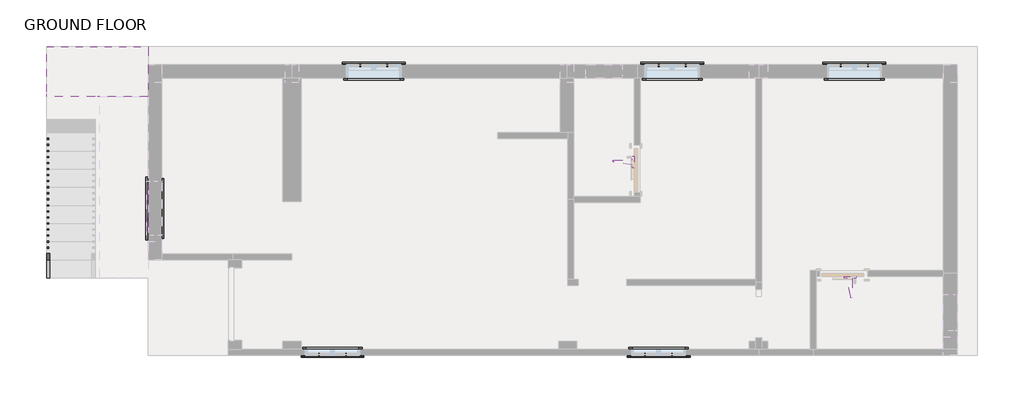
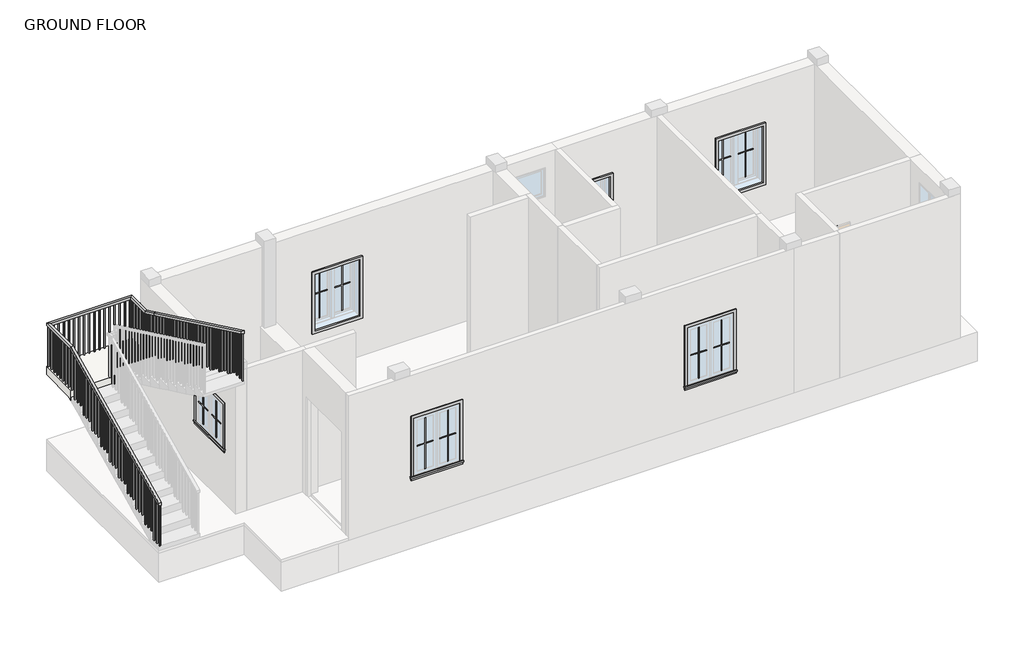
# One storey, part 3 of 3: 26 proxies, 1 railing, 1 slab.
"""IFC4 building model written with IfcOpenShell, lengths in millimetres."""

from ifc_helpers import new_model, si_unit, frame, origin, place, context, project, spatial, polyline, outline, extrude, faceted_brep, transform, mapped, element, save
from components import bel_door_closer_bel_door_closer_f210e2f3, bel_door_closer_bel_door_closer_a3520c2f, muntin_pattern_2x2_muntin_pattern_2x2_1acec82f, muntin_pattern_2x2_muntin_pattern_2x2_43d02eee, muntin_pattern_2x2_muntin_pattern_2x2_d1c6e638, muntin_pattern_2x2_muntin_pattern_2x2_37b95fb2, trim_window_exterior_flat_with_sill_e4b28ec3, trim_window_exterior_flat_with_sill_84e24481, trim_window_interior_flat_picture_frame_39ff4276, trim_window_interior_flat_picture_frame_28d4e5dc

model = new_model("IFC4")

# Units and contexts
model_context = context("Model", 3, world=origin())
ifc_project = project(units=[si_unit("LENGTHUNIT", "METRE", prefix="MILLI")], contexts=[model_context])

# Site, building, storey
site = spatial("IfcSite", under=ifc_project)
building = spatial("IfcBuilding", under=site)
storey = spatial("IfcBuildingStorey", under=building, Name="GROUND FLOOR", Elevation=0.0)

# Proxies
placement = place(None, origin())
bel_door_closer_bel_door_closer_shape = bel_door_closer_bel_door_closer_f210e2f3(model_context)
element("IfcBuildingElementProxy", 1, Name="BEL-Door Closer : BEL-Door Closer", ObjectType="BEL-Door Closer : BEL-Door Closer", at=placement, inside=storey, context=model_context, shape_type="MappedRepresentation", body=[
    mapped(bel_door_closer_bel_door_closer_shape, transform((6826.3533773, 1546.5642852, 2144.6957985), x_axis=(-1.0, 0.0, 0.0), y_axis=(0.0, 0.0, -1.0), z_axis=(0.0, -1.0, 0.0))),
])
bel_door_closer_bel_door_closer_2_shape = bel_door_closer_bel_door_closer_a3520c2f(model_context)
element("IfcBuildingElementProxy", 2, Name="BEL-Door Closer : BEL-Door Closer", ObjectType="BEL-Door Closer : BEL-Door Closer", at=placement, inside=storey, context=model_context, shape_type="MappedRepresentation", body=[
    mapped(bel_door_closer_bel_door_closer_2_shape, transform((3460.0408773, 3211.0767852, 2144.6957985), x_axis=(0.0, -1.0, 0.0), y_axis=(0.0, 0.0, 1.0), z_axis=(-1.0, 0.0, 0.0))),
])
muntin_pattern_2x2_muntin_pattern_2x2_shape = muntin_pattern_2x2_muntin_pattern_2x2_1acec82f(model_context)
element("IfcBuildingElementProxy", 3, Name="Muntin Pattern_2x2 : Muntin Pattern_2x2", ObjectType="Muntin Pattern_2x2 : Muntin Pattern_2x2", at=placement, inside=storey, context=model_context, shape_type="MappedRepresentation", body=[
    mapped(muntin_pattern_2x2_muntin_pattern_2x2_shape, transform((-1135.7716227, 5093.0392852, 984.25), x_axis=(1.0, 0.0, 0.0), y_axis=(0.0, 1.0, 0.0), z_axis=(0.0, 0.0, 1.0))),
])
element("IfcBuildingElementProxy", 4, Name="Muntin Pattern_2x2 : Muntin Pattern_2x2", ObjectType="Muntin Pattern_2x2 : Muntin Pattern_2x2", at=placement, inside=storey, context=model_context, shape_type="MappedRepresentation", body=[
    mapped(muntin_pattern_2x2_muntin_pattern_2x2_shape, transform((3868.0283773, 5093.0392852, 984.25), x_axis=(1.0, 0.0, 0.0), y_axis=(0.0, 1.0, 0.0), z_axis=(0.0, 0.0, 1.0))),
])
element("IfcBuildingElementProxy", 5, Name="Muntin Pattern_2x2 : Muntin Pattern_2x2", ObjectType="Muntin Pattern_2x2 : Muntin Pattern_2x2", at=placement, inside=storey, context=model_context, shape_type="MappedRepresentation", body=[
    mapped(muntin_pattern_2x2_muntin_pattern_2x2_shape, transform((6922.3783773, 5093.0392852, 984.25), x_axis=(1.0, 0.0, 0.0), y_axis=(0.0, 1.0, 0.0), z_axis=(0.0, 0.0, 1.0))),
])
element("IfcBuildingElementProxy", 6, Name="Muntin Pattern_2x2 : Muntin Pattern_2x2", ObjectType="Muntin Pattern_2x2 : Muntin Pattern_2x2", at=placement, inside=storey, context=model_context, shape_type="MappedRepresentation", body=[
    mapped(muntin_pattern_2x2_muntin_pattern_2x2_shape, transform((4093.4533773, 235.2892852, 984.25), x_axis=(-1.0, 0.0, 0.0), y_axis=(0.0, -1.0, 0.0), z_axis=(0.0, 0.0, 1.0))),
])
element("IfcBuildingElementProxy", 7, Name="Muntin Pattern_2x2 : Muntin Pattern_2x2", ObjectType="Muntin Pattern_2x2 : Muntin Pattern_2x2", at=placement, inside=storey, context=model_context, shape_type="MappedRepresentation", body=[
    mapped(muntin_pattern_2x2_muntin_pattern_2x2_shape, transform((-1373.8966227, 235.2892852, 984.25), x_axis=(-1.0, 0.0, 0.0), y_axis=(0.0, -1.0, 0.0), z_axis=(0.0, 0.0, 1.0))),
])
muntin_pattern_2x2_muntin_pattern_2x2_2_shape = muntin_pattern_2x2_muntin_pattern_2x2_43d02eee(model_context)
element("IfcBuildingElementProxy", 8, Name="Muntin Pattern_2x2 : Muntin Pattern_2x2", ObjectType="Muntin Pattern_2x2 : Muntin Pattern_2x2", at=placement, inside=storey, context=model_context, shape_type="MappedRepresentation", body=[
    mapped(muntin_pattern_2x2_muntin_pattern_2x2_2_shape, transform((-681.7466227, 5093.0392852, 984.25), x_axis=(-1.0, 0.0, 0.0), y_axis=(0.0, -1.0, 0.0), z_axis=(0.0, 0.0, 1.0))),
])
element("IfcBuildingElementProxy", 9, Name="Muntin Pattern_2x2 : Muntin Pattern_2x2", ObjectType="Muntin Pattern_2x2 : Muntin Pattern_2x2", at=placement, inside=storey, context=model_context, shape_type="MappedRepresentation", body=[
    mapped(muntin_pattern_2x2_muntin_pattern_2x2_2_shape, transform((4322.0533773, 5093.0392852, 984.25), x_axis=(-1.0, 0.0, 0.0), y_axis=(0.0, -1.0, 0.0), z_axis=(0.0, 0.0, 1.0))),
])
element("IfcBuildingElementProxy", 10, Name="Muntin Pattern_2x2 : Muntin Pattern_2x2", ObjectType="Muntin Pattern_2x2 : Muntin Pattern_2x2", at=placement, inside=storey, context=model_context, shape_type="MappedRepresentation", body=[
    mapped(muntin_pattern_2x2_muntin_pattern_2x2_2_shape, transform((7376.4033773, 5093.0392852, 984.25), x_axis=(-1.0, 0.0, 0.0), y_axis=(0.0, -1.0, 0.0), z_axis=(0.0, 0.0, 1.0))),
])
element("IfcBuildingElementProxy", 11, Name="Muntin Pattern_2x2 : Muntin Pattern_2x2", ObjectType="Muntin Pattern_2x2 : Muntin Pattern_2x2", at=placement, inside=storey, context=model_context, shape_type="MappedRepresentation", body=[
    mapped(muntin_pattern_2x2_muntin_pattern_2x2_2_shape, transform((3639.4283773, 235.2892852, 984.25), x_axis=(1.0, 0.0, 0.0), y_axis=(0.0, 1.0, 0.0), z_axis=(0.0, 0.0, 1.0))),
])
element("IfcBuildingElementProxy", 12, Name="Muntin Pattern_2x2 : Muntin Pattern_2x2", ObjectType="Muntin Pattern_2x2 : Muntin Pattern_2x2", at=placement, inside=storey, context=model_context, shape_type="MappedRepresentation", body=[
    mapped(muntin_pattern_2x2_muntin_pattern_2x2_2_shape, transform((-1827.9216227, 235.2892852, 984.25), x_axis=(1.0, 0.0, 0.0), y_axis=(0.0, 1.0, 0.0), z_axis=(0.0, 0.0, 1.0))),
])
muntin_pattern_2x2_muntin_pattern_2x2_3_shape = muntin_pattern_2x2_muntin_pattern_2x2_d1c6e638(model_context)
element("IfcBuildingElementProxy", 13, Name="Muntin Pattern_2x2 : Muntin Pattern_2x2", ObjectType="Muntin Pattern_2x2 : Muntin Pattern_2x2", at=placement, inside=storey, context=model_context, shape_type="MappedRepresentation", body=[
    mapped(muntin_pattern_2x2_muntin_pattern_2x2_3_shape, transform((-4683.8341227, 2462.5517852, 1289.05), x_axis=(0.0, 1.0, 0.0), y_axis=(-1.0, 0.0, 0.0), z_axis=(0.0, 0.0, 1.0))),
])
muntin_pattern_2x2_muntin_pattern_2x2_4_shape = muntin_pattern_2x2_muntin_pattern_2x2_37b95fb2(model_context)
element("IfcBuildingElementProxy", 14, Name="Muntin Pattern_2x2 : Muntin Pattern_2x2", ObjectType="Muntin Pattern_2x2 : Muntin Pattern_2x2", at=placement, inside=storey, context=model_context, shape_type="MappedRepresentation", body=[
    mapped(muntin_pattern_2x2_muntin_pattern_2x2_4_shape, transform((-4683.8341227, 2916.5767852, 1289.05), x_axis=(0.0, -1.0, 0.0), y_axis=(1.0, 0.0, 0.0), z_axis=(0.0, 0.0, 1.0))),
])
trim_window_exterior_flat_with_sill_shape = trim_window_exterior_flat_with_sill_e4b28ec3(model_context)
element("IfcBuildingElementProxy", 15, Name="Trim-Window-Exterior-Flat : with Sill", ObjectType="Trim-Window-Exterior-Flat : with Sill", at=placement, inside=storey, context=model_context, shape_type="MappedRepresentation", body=[
    mapped(trim_window_exterior_flat_with_sill_shape, transform((-908.7591227, 5102.5642852, 2133.6), x_axis=(-1.0, 0.0, 0.0), y_axis=(0.0, 0.0, 1.0), z_axis=(0.0, 1.0, 0.0))),
])
element("IfcBuildingElementProxy", 16, Name="Trim-Window-Exterior-Flat : with Sill", ObjectType="Trim-Window-Exterior-Flat : with Sill", at=placement, inside=storey, context=model_context, shape_type="MappedRepresentation", body=[
    mapped(trim_window_exterior_flat_with_sill_shape, transform((4095.0408773, 5102.5642852, 2133.6), x_axis=(-1.0, 0.0, 0.0), y_axis=(0.0, 0.0, 1.0), z_axis=(0.0, 1.0, 0.0))),
])
element("IfcBuildingElementProxy", 17, Name="Trim-Window-Exterior-Flat : with Sill", ObjectType="Trim-Window-Exterior-Flat : with Sill", at=placement, inside=storey, context=model_context, shape_type="MappedRepresentation", body=[
    mapped(trim_window_exterior_flat_with_sill_shape, transform((7149.3908773, 5102.5642852, 2133.6), x_axis=(-1.0, 0.0, 0.0), y_axis=(0.0, 0.0, 1.0), z_axis=(0.0, 1.0, 0.0))),
])
element("IfcBuildingElementProxy", 18, Name="Trim-Window-Exterior-Flat : with Sill", ObjectType="Trim-Window-Exterior-Flat : with Sill", at=placement, inside=storey, context=model_context, shape_type="MappedRepresentation", body=[
    mapped(trim_window_exterior_flat_with_sill_shape, transform((3866.4408773, 225.7642852, 2133.6), x_axis=(1.0, 0.0, 0.0), y_axis=(0.0, 0.0, 1.0), z_axis=(0.0, -1.0, 0.0))),
])
element("IfcBuildingElementProxy", 19, Name="Trim-Window-Exterior-Flat : with Sill", ObjectType="Trim-Window-Exterior-Flat : with Sill", at=placement, inside=storey, context=model_context, shape_type="MappedRepresentation", body=[
    mapped(trim_window_exterior_flat_with_sill_shape, transform((-1600.9091227, 225.7642852, 2133.6), x_axis=(1.0, 0.0, 0.0), y_axis=(0.0, 0.0, 1.0), z_axis=(0.0, -1.0, 0.0))),
])
trim_window_exterior_flat_with_sill_2_shape = trim_window_exterior_flat_with_sill_84e24481(model_context)
element("IfcBuildingElementProxy", 20, Name="Trim-Window-Exterior-Flat : with Sill", ObjectType="Trim-Window-Exterior-Flat : with Sill", at=placement, inside=storey, context=model_context, shape_type="MappedRepresentation", body=[
    mapped(trim_window_exterior_flat_with_sill_2_shape, transform((-4693.3591227, 2689.5642852, 2133.6), x_axis=(0.0, -1.0, 0.0), y_axis=(0.0, 0.0, 1.0), z_axis=(-1.0, 0.0, 0.0))),
])
trim_window_interior_flat_picture_frame_shape = trim_window_interior_flat_picture_frame_39ff4276(model_context)
element("IfcBuildingElementProxy", 21, Name="Trim-Window-Interior-Flat : Picture Frame", ObjectType="Trim-Window-Interior-Flat : Picture Frame", at=placement, inside=storey, context=model_context, shape_type="MappedRepresentation", body=[
    mapped(trim_window_interior_flat_picture_frame_shape, transform((-908.7591227, 4873.9642852, 2133.6), x_axis=(1.0, 0.0, 0.0), y_axis=(0.0, 0.0, 1.0), z_axis=(0.0, -1.0, 0.0))),
])
element("IfcBuildingElementProxy", 22, Name="Trim-Window-Interior-Flat : Picture Frame", ObjectType="Trim-Window-Interior-Flat : Picture Frame", at=placement, inside=storey, context=model_context, shape_type="MappedRepresentation", body=[
    mapped(trim_window_interior_flat_picture_frame_shape, transform((4095.0408773, 4873.9642852, 2133.6), x_axis=(1.0, 0.0, 0.0), y_axis=(0.0, 0.0, 1.0), z_axis=(0.0, -1.0, 0.0))),
])
element("IfcBuildingElementProxy", 23, Name="Trim-Window-Interior-Flat : Picture Frame", ObjectType="Trim-Window-Interior-Flat : Picture Frame", at=placement, inside=storey, context=model_context, shape_type="MappedRepresentation", body=[
    mapped(trim_window_interior_flat_picture_frame_shape, transform((7149.3908773, 4873.9642852, 2133.6), x_axis=(1.0, 0.0, 0.0), y_axis=(0.0, 0.0, 1.0), z_axis=(0.0, -1.0, 0.0))),
])
element("IfcBuildingElementProxy", 24, Name="Trim-Window-Interior-Flat : Picture Frame", ObjectType="Trim-Window-Interior-Flat : Picture Frame", at=placement, inside=storey, context=model_context, shape_type="MappedRepresentation", body=[
    mapped(trim_window_interior_flat_picture_frame_shape, transform((3866.4408773, 327.3642852, 2133.6), x_axis=(-1.0, 0.0, 0.0), y_axis=(0.0, 0.0, 1.0), z_axis=(0.0, 1.0, 0.0))),
])
element("IfcBuildingElementProxy", 25, Name="Trim-Window-Interior-Flat : Picture Frame", ObjectType="Trim-Window-Interior-Flat : Picture Frame", at=placement, inside=storey, context=model_context, shape_type="MappedRepresentation", body=[
    mapped(trim_window_interior_flat_picture_frame_shape, transform((-1600.9091227, 327.3642852, 2133.6), x_axis=(-1.0, 0.0, 0.0), y_axis=(0.0, 0.0, 1.0), z_axis=(0.0, 1.0, 0.0))),
])
trim_window_interior_flat_picture_frame_2_shape = trim_window_interior_flat_picture_frame_28d4e5dc(model_context)
element("IfcBuildingElementProxy", 26, Name="Trim-Window-Interior-Flat : Picture Frame", ObjectType="Trim-Window-Interior-Flat : Picture Frame", at=placement, inside=storey, context=model_context, shape_type="MappedRepresentation", body=[
    mapped(trim_window_interior_flat_picture_frame_2_shape, transform((-4464.7591227, 2689.5642852, 2133.6), x_axis=(0.0, 1.0, 0.0), y_axis=(0.0, 0.0, 1.0), z_axis=(1.0, 0.0, 0.0))),
])

# Railing
element("IfcRailing", 27, ObjectType="Handrail - Rectangular", at=placement, inside=storey, context=model_context, shape_type="SolidModel", body=[
    faceted_brep([(-6395.1591227, 1521.1642852, 1059.8727273), (-6395.1591227, 1521.1642852, 1003.5834559), (-6344.3591227, 1521.1642852, 1003.5834559), (-6344.3591227, 1521.1642852, 1059.8727273), (-6395.1591227, 4569.1642852, 2514.6), (-6395.1591227, 4580.6656156, 2463.8), (-6344.3591227, 4580.6656156, 2463.8), (-6344.3591227, 4569.1642852, 2514.6), (-6395.1591227, 5407.3642852, 2514.6), (-6395.1591227, 5407.3642852, 2463.8), (-6344.3591227, 5356.5642852, 2463.8), (-6344.3591227, 5356.5642852, 2514.6), (-4693.3591227, 5407.3642852, 2514.6), (-4693.3591227, 5407.3642852, 2463.8), (-4744.1591227, 5356.5642852, 2463.8), (-4744.1591227, 5356.5642852, 2514.6), (-4693.3591227, 4873.9642852, 2514.6), (-4693.3591227, 4862.4629548, 2463.8), (-4744.1591227, 4862.4629548, 2463.8), (-4744.1591227, 4873.9642852, 2514.6), (-4693.3591227, 4569.1642852, 2660.0727273), (-4693.3591227, 4547.2832222, 2614.2266906), (-4744.1591227, 4547.2832222, 2614.2266906), (-4744.1591227, 4569.1642852, 2660.0727273), (-4693.3591227, 1521.1642852, 4114.8), (-4744.1591227, 1521.1642852, 4114.8), (-4744.1591227, 1521.1642852, 4058.5107287), (-4693.3591227, 1521.1642852, 4058.5107287)], [[[0, 1, 2, 3]], [[1, 0, 4, 5]], [[2, 1, 5, 6]], [[3, 2, 6, 7]], [[0, 3, 7, 4]], [[5, 4, 8, 9]], [[6, 5, 9, 10]], [[7, 6, 10, 11]], [[4, 7, 11, 8]], [[9, 8, 12, 13]], [[10, 9, 13, 14]], [[11, 10, 14, 15]], [[8, 11, 15, 12]], [[13, 12, 16, 17]], [[14, 13, 17, 18]], [[15, 14, 18, 19]], [[12, 15, 19, 16]], [[17, 16, 20, 21]], [[18, 17, 21, 22]], [[19, 18, 22, 23]], [[16, 19, 23, 20]], [[24, 25, 26, 27]], [[21, 20, 24, 27]], [[22, 21, 27, 26]], [[23, 22, 26, 25]], [[20, 23, 25, 24]]]),
    extrude(outline(polyline([(1632.2892852, 4005.4737969), (1632.2892852, 3054.9272727), (1613.2392852, 3054.9272727), (1613.2392852, 4014.5658423), (1632.2892852, 4005.4737969)])), frame((-4728.2841227, 0.0, 0.0), z_axis=(1.0, 0.0, 0.0), x_axis=(0.0, 1.0, 0.0)), (0.0, 0.0, 1.0), 19.05),
    extrude(outline(polyline([(1733.8892852, 3956.9828878), (1733.8892852, 3054.9272727), (1714.8392852, 3054.9272727), (1714.8392852, 3966.0749332), (1733.8892852, 3956.9828878)])), frame((-4728.2841227, 0.0, 0.0), z_axis=(1.0, 0.0, 0.0), x_axis=(0.0, 1.0, 0.0)), (0.0, 0.0, 1.0), 19.05),
    extrude(outline(polyline([(1835.4892852, 3908.4919787), (1835.4892852, 3054.9272727), (1816.4392852, 3054.9272727), (1816.4392852, 3917.5840241), (1835.4892852, 3908.4919787)])), frame((-4728.2841227, 0.0, 0.0), z_axis=(1.0, 0.0, 0.0), x_axis=(0.0, 1.0, 0.0)), (0.0, 0.0, 1.0), 19.05),
    extrude(outline(polyline([(1937.0892852, 3860.0010696), (1937.0892852, 2909.4545455), (1918.0392852, 2909.4545455), (1918.0392852, 3869.093115), (1937.0892852, 3860.0010696)])), frame((-4728.2841227, 0.0, 0.0), z_axis=(1.0, 0.0, 0.0), x_axis=(0.0, 1.0, 0.0)), (0.0, 0.0, 1.0), 19.05),
    extrude(outline(polyline([(2038.6892852, 3811.5101605), (2038.6892852, 2909.4545455), (2019.6392852, 2909.4545455), (2019.6392852, 3820.6022059), (2038.6892852, 3811.5101605)])), frame((-4728.2841227, 0.0, 0.0), z_axis=(1.0, 0.0, 0.0), x_axis=(0.0, 1.0, 0.0)), (0.0, 0.0, 1.0), 19.05),
    extrude(outline(polyline([(2140.2892852, 3763.0192514), (2140.2892852, 2909.4545455), (2121.2392852, 2909.4545455), (2121.2392852, 3772.1112969), (2140.2892852, 3763.0192514)])), frame((-4728.2841227, 0.0, 0.0), z_axis=(1.0, 0.0, 0.0), x_axis=(0.0, 1.0, 0.0)), (0.0, 0.0, 1.0), 19.05),
    extrude(outline(polyline([(2241.8892852, 3714.5283423), (2241.8892852, 2763.9818182), (2222.8392852, 2763.9818182), (2222.8392852, 3723.6203878), (2241.8892852, 3714.5283423)])), frame((-4728.2841227, 0.0, 0.0), z_axis=(1.0, 0.0, 0.0), x_axis=(0.0, 1.0, 0.0)), (0.0, 0.0, 1.0), 19.05),
    extrude(outline(polyline([(2343.4892852, 3666.0374332), (2343.4892852, 2763.9818182), (2324.4392852, 2763.9818182), (2324.4392852, 3675.1294787), (2343.4892852, 3666.0374332)])), frame((-4728.2841227, 0.0, 0.0), z_axis=(1.0, 0.0, 0.0), x_axis=(0.0, 1.0, 0.0)), (0.0, 0.0, 1.0), 19.05),
    extrude(outline(polyline([(2445.0892852, 3617.5465241), (2445.0892852, 2763.9818182), (2426.0392852, 2763.9818182), (2426.0392852, 3626.6385696), (2445.0892852, 3617.5465241)])), frame((-4728.2841227, 0.0, 0.0), z_axis=(1.0, 0.0, 0.0), x_axis=(0.0, 1.0, 0.0)), (0.0, 0.0, 1.0), 19.05),
    extrude(outline(polyline([(2546.6892852, 3569.055615), (2546.6892852, 2618.5090909), (2527.6392852, 2618.5090909), (2527.6392852, 3578.1476605), (2546.6892852, 3569.055615)])), frame((-4728.2841227, 0.0, 0.0), z_axis=(1.0, 0.0, 0.0), x_axis=(0.0, 1.0, 0.0)), (0.0, 0.0, 1.0), 19.05),
    extrude(outline(polyline([(2648.2892852, 3520.5647059), (2648.2892852, 2618.5090909), (2629.2392852, 2618.5090909), (2629.2392852, 3529.6567514), (2648.2892852, 3520.5647059)])), frame((-4728.2841227, 0.0, 0.0), z_axis=(1.0, 0.0, 0.0), x_axis=(0.0, 1.0, 0.0)), (0.0, 0.0, 1.0), 19.05),
    extrude(outline(polyline([(2749.8892852, 3472.0737969), (2749.8892852, 2618.5090909), (2730.8392852, 2618.5090909), (2730.8392852, 3481.1658423), (2749.8892852, 3472.0737969)])), frame((-4728.2841227, 0.0, 0.0), z_axis=(1.0, 0.0, 0.0), x_axis=(0.0, 1.0, 0.0)), (0.0, 0.0, 1.0), 19.05),
    extrude(outline(polyline([(2851.4892852, 3423.5828878), (2851.4892852, 2473.0363636), (2832.4392852, 2473.0363636), (2832.4392852, 3432.6749332), (2851.4892852, 3423.5828878)])), frame((-4728.2841227, 0.0, 0.0), z_axis=(1.0, 0.0, 0.0), x_axis=(0.0, 1.0, 0.0)), (0.0, 0.0, 1.0), 19.05),
    extrude(outline(polyline([(2953.0892852, 3375.0919787), (2953.0892852, 2473.0363636), (2934.0392852, 2473.0363636), (2934.0392852, 3384.1840241), (2953.0892852, 3375.0919787)])), frame((-4728.2841227, 0.0, 0.0), z_axis=(1.0, 0.0, 0.0), x_axis=(0.0, 1.0, 0.0)), (0.0, 0.0, 1.0), 19.05),
    extrude(outline(polyline([(3054.6892852, 3326.6010696), (3054.6892852, 2473.0363636), (3035.6392852, 2473.0363636), (3035.6392852, 3335.693115), (3054.6892852, 3326.6010696)])), frame((-4728.2841227, 0.0, 0.0), z_axis=(1.0, 0.0, 0.0), x_axis=(0.0, 1.0, 0.0)), (0.0, 0.0, 1.0), 19.05),
    extrude(outline(polyline([(3156.2892852, 3278.1101605), (3156.2892852, 2327.5636364), (3137.2392852, 2327.5636364), (3137.2392852, 3287.2022059), (3156.2892852, 3278.1101605)])), frame((-4728.2841227, 0.0, 0.0), z_axis=(1.0, 0.0, 0.0), x_axis=(0.0, 1.0, 0.0)), (0.0, 0.0, 1.0), 19.05),
    extrude(outline(polyline([(3257.8892852, 3229.6192514), (3257.8892852, 2327.5636364), (3238.8392852, 2327.5636364), (3238.8392852, 3238.7112969), (3257.8892852, 3229.6192514)])), frame((-4728.2841227, 0.0, 0.0), z_axis=(1.0, 0.0, 0.0), x_axis=(0.0, 1.0, 0.0)), (0.0, 0.0, 1.0), 19.05),
    extrude(outline(polyline([(3359.4892852, 3181.1283423), (3359.4892852, 2327.5636364), (3340.4392852, 2327.5636364), (3340.4392852, 3190.2203878), (3359.4892852, 3181.1283423)])), frame((-4728.2841227, 0.0, 0.0), z_axis=(1.0, 0.0, 0.0), x_axis=(0.0, 1.0, 0.0)), (0.0, 0.0, 1.0), 19.05),
    extrude(outline(polyline([(3461.0892852, 3132.6374332), (3461.0892852, 2182.0909091), (3442.0392852, 2182.0909091), (3442.0392852, 3141.7294787), (3461.0892852, 3132.6374332)])), frame((-4728.2841227, 0.0, 0.0), z_axis=(1.0, 0.0, 0.0), x_axis=(0.0, 1.0, 0.0)), (0.0, 0.0, 1.0), 19.05),
    extrude(outline(polyline([(3562.6892852, 3084.1465241), (3562.6892852, 2182.0909091), (3543.6392852, 2182.0909091), (3543.6392852, 3093.2385696), (3562.6892852, 3084.1465241)])), frame((-4728.2841227, 0.0, 0.0), z_axis=(1.0, 0.0, 0.0), x_axis=(0.0, 1.0, 0.0)), (0.0, 0.0, 1.0), 19.05),
    extrude(outline(polyline([(3664.2892852, 3035.655615), (3664.2892852, 2182.0909091), (3645.2392852, 2182.0909091), (3645.2392852, 3044.7476605), (3664.2892852, 3035.655615)])), frame((-4728.2841227, 0.0, 0.0), z_axis=(1.0, 0.0, 0.0), x_axis=(0.0, 1.0, 0.0)), (0.0, 0.0, 1.0), 19.05),
    extrude(outline(polyline([(3765.8892852, 2987.1647059), (3765.8892852, 2036.6181818), (3746.8392852, 2036.6181818), (3746.8392852, 2996.2567514), (3765.8892852, 2987.1647059)])), frame((-4728.2841227, 0.0, 0.0), z_axis=(1.0, 0.0, 0.0), x_axis=(0.0, 1.0, 0.0)), (0.0, 0.0, 1.0), 19.05),
    extrude(outline(polyline([(3867.4892852, 2938.6737969), (3867.4892852, 2036.6181818), (3848.4392852, 2036.6181818), (3848.4392852, 2947.7658423), (3867.4892852, 2938.6737969)])), frame((-4728.2841227, 0.0, 0.0), z_axis=(1.0, 0.0, 0.0), x_axis=(0.0, 1.0, 0.0)), (0.0, 0.0, 1.0), 19.05),
    extrude(outline(polyline([(3969.0892852, 2890.1828878), (3969.0892852, 2036.6181818), (3950.0392852, 2036.6181818), (3950.0392852, 2899.2749332), (3969.0892852, 2890.1828878)])), frame((-4728.2841227, 0.0, 0.0), z_axis=(1.0, 0.0, 0.0), x_axis=(0.0, 1.0, 0.0)), (0.0, 0.0, 1.0), 19.05),
    extrude(outline(polyline([(4070.6892852, 2841.6919787), (4070.6892852, 1891.1454545), (4051.6392852, 1891.1454545), (4051.6392852, 2850.7840241), (4070.6892852, 2841.6919787)])), frame((-4728.2841227, 0.0, 0.0), z_axis=(1.0, 0.0, 0.0), x_axis=(0.0, 1.0, 0.0)), (0.0, 0.0, 1.0), 19.05),
    extrude(outline(polyline([(4172.2892852, 2793.2010696), (4172.2892852, 1891.1454545), (4153.2392852, 1891.1454545), (4153.2392852, 2802.293115), (4172.2892852, 2793.2010696)])), frame((-4728.2841227, 0.0, 0.0), z_axis=(1.0, 0.0, 0.0), x_axis=(0.0, 1.0, 0.0)), (0.0, 0.0, 1.0), 19.05),
    extrude(outline(polyline([(4273.8892852, 2744.7101605), (4273.8892852, 1891.1454545), (4254.8392852, 1891.1454545), (4254.8392852, 2753.8022059), (4273.8892852, 2744.7101605)])), frame((-4728.2841227, 0.0, 0.0), z_axis=(1.0, 0.0, 0.0), x_axis=(0.0, 1.0, 0.0)), (0.0, 0.0, 1.0), 19.05),
    extrude(outline(polyline([(4375.4892852, 2696.2192514), (4375.4892852, 1745.6727273), (4356.4392852, 1745.6727273), (4356.4392852, 2705.3112969), (4375.4892852, 2696.2192514)])), frame((-4728.2841227, 0.0, 0.0), z_axis=(1.0, 0.0, 0.0), x_axis=(0.0, 1.0, 0.0)), (0.0, 0.0, 1.0), 19.05),
    extrude(outline(polyline([(4477.0892852, 2647.7283423), (4477.0892852, 1745.6727273), (4458.0392852, 1745.6727273), (4458.0392852, 2656.8203878), (4477.0892852, 2647.7283423)])), frame((-4728.2841227, 0.0, 0.0), z_axis=(1.0, 0.0, 0.0), x_axis=(0.0, 1.0, 0.0)), (0.0, 0.0, 1.0), 19.05),
    extrude(outline(polyline([(4680.2892852, 2550.7465241), (4680.2892852, 1600.2), (4661.2392852, 1600.2), (4661.2392852, 2559.8385696), (4680.2892852, 2550.7465241)])), frame((-4728.2841227, 0.0, 0.0), z_axis=(1.0, 0.0, 0.0), x_axis=(0.0, 1.0, 0.0)), (0.0, 0.0, 1.0), 19.05),
    extrude(outline(polyline([(4781.8892852, 2502.255615), (4781.8892852, 1600.2), (4762.8392852, 1600.2), (4762.8392852, 2511.3476605), (4781.8892852, 2502.255615)])), frame((-4728.2841227, 0.0, 0.0), z_axis=(1.0, 0.0, 0.0), x_axis=(0.0, 1.0, 0.0)), (0.0, 0.0, 1.0), 19.05),
    extrude(outline(polyline([(-4709.2341227, 4883.4892852), (-4709.2341227, 4864.4392852), (-4728.2841227, 4864.4392852), (-4728.2841227, 4883.4892852), (-4709.2341227, 4883.4892852)])), frame((0.0, 0.0, 1600.2), z_axis=(0.0, 0.0, 1.0), x_axis=(1.0, 0.0, 0.0)), (0.0, 0.0, 1.0), 863.6),
    extrude(outline(polyline([(-4709.2341227, 4985.0892852), (-4709.2341227, 4966.0392852), (-4728.2841227, 4966.0392852), (-4728.2841227, 4985.0892852), (-4709.2341227, 4985.0892852)])), frame((0.0, 0.0, 1600.2), z_axis=(0.0, 0.0, 1.0), x_axis=(1.0, 0.0, 0.0)), (0.0, 0.0, 1.0), 863.6),
    extrude(outline(polyline([(-4709.2341227, 5086.6892852), (-4709.2341227, 5067.6392852), (-4728.2841227, 5067.6392852), (-4728.2841227, 5086.6892852), (-4709.2341227, 5086.6892852)])), frame((0.0, 0.0, 1600.2), z_axis=(0.0, 0.0, 1.0), x_axis=(1.0, 0.0, 0.0)), (0.0, 0.0, 1.0), 863.6),
    extrude(outline(polyline([(-4709.2341227, 5188.2892852), (-4709.2341227, 5169.2392852), (-4728.2841227, 5169.2392852), (-4728.2841227, 5188.2892852), (-4709.2341227, 5188.2892852)])), frame((0.0, 0.0, 1600.2), z_axis=(0.0, 0.0, 1.0), x_axis=(1.0, 0.0, 0.0)), (0.0, 0.0, 1.0), 863.6),
    extrude(outline(polyline([(-4709.2341227, 5289.8892852), (-4709.2341227, 5270.8392852), (-4728.2841227, 5270.8392852), (-4728.2841227, 5289.8892852), (-4709.2341227, 5289.8892852)])), frame((0.0, 0.0, 1600.2), z_axis=(0.0, 0.0, 1.0), x_axis=(1.0, 0.0, 0.0)), (0.0, 0.0, 1.0), 863.6),
    extrude(outline(polyline([(-4753.6841227, 5391.4892852), (-4734.6341227, 5391.4892852), (-4734.6341227, 5372.4392852), (-4753.6841227, 5372.4392852), (-4753.6841227, 5391.4892852)])), frame((0.0, 0.0, 1600.2), z_axis=(0.0, 0.0, 1.0), x_axis=(1.0, 0.0, 0.0)), (0.0, 0.0, 1.0), 863.6),
    extrude(outline(polyline([(-4855.2841227, 5391.4892852), (-4836.2341227, 5391.4892852), (-4836.2341227, 5372.4392852), (-4855.2841227, 5372.4392852), (-4855.2841227, 5391.4892852)])), frame((0.0, 0.0, 1600.2), z_axis=(0.0, 0.0, 1.0), x_axis=(1.0, 0.0, 0.0)), (0.0, 0.0, 1.0), 863.6),
    extrude(outline(polyline([(-4956.8841227, 5391.4892852), (-4937.8341227, 5391.4892852), (-4937.8341227, 5372.4392852), (-4956.8841227, 5372.4392852), (-4956.8841227, 5391.4892852)])), frame((0.0, 0.0, 1600.2), z_axis=(0.0, 0.0, 1.0), x_axis=(1.0, 0.0, 0.0)), (0.0, 0.0, 1.0), 863.6),
    extrude(outline(polyline([(-5058.4841227, 5391.4892852), (-5039.4341227, 5391.4892852), (-5039.4341227, 5372.4392852), (-5058.4841227, 5372.4392852), (-5058.4841227, 5391.4892852)])), frame((0.0, 0.0, 1600.2), z_axis=(0.0, 0.0, 1.0), x_axis=(1.0, 0.0, 0.0)), (0.0, 0.0, 1.0), 863.6),
    extrude(outline(polyline([(-5160.0841227, 5391.4892852), (-5141.0341227, 5391.4892852), (-5141.0341227, 5372.4392852), (-5160.0841227, 5372.4392852), (-5160.0841227, 5391.4892852)])), frame((0.0, 0.0, 1600.2), z_axis=(0.0, 0.0, 1.0), x_axis=(1.0, 0.0, 0.0)), (0.0, 0.0, 1.0), 863.6),
    extrude(outline(polyline([(-5261.6841227, 5391.4892852), (-5242.6341227, 5391.4892852), (-5242.6341227, 5372.4392852), (-5261.6841227, 5372.4392852), (-5261.6841227, 5391.4892852)])), frame((0.0, 0.0, 1600.2), z_axis=(0.0, 0.0, 1.0), x_axis=(1.0, 0.0, 0.0)), (0.0, 0.0, 1.0), 863.6),
    extrude(outline(polyline([(-5363.2841227, 5391.4892852), (-5344.2341227, 5391.4892852), (-5344.2341227, 5372.4392852), (-5363.2841227, 5372.4392852), (-5363.2841227, 5391.4892852)])), frame((0.0, 0.0, 1600.2), z_axis=(0.0, 0.0, 1.0), x_axis=(1.0, 0.0, 0.0)), (0.0, 0.0, 1.0), 863.6),
    extrude(outline(polyline([(-5464.8841227, 5391.4892852), (-5445.8341227, 5391.4892852), (-5445.8341227, 5372.4392852), (-5464.8841227, 5372.4392852), (-5464.8841227, 5391.4892852)])), frame((0.0, 0.0, 1600.2), z_axis=(0.0, 0.0, 1.0), x_axis=(1.0, 0.0, 0.0)), (0.0, 0.0, 1.0), 863.6),
    extrude(outline(polyline([(-5566.4841227, 5391.4892852), (-5547.4341227, 5391.4892852), (-5547.4341227, 5372.4392852), (-5566.4841227, 5372.4392852), (-5566.4841227, 5391.4892852)])), frame((0.0, 0.0, 1600.2), z_axis=(0.0, 0.0, 1.0), x_axis=(1.0, 0.0, 0.0)), (0.0, 0.0, 1.0), 863.6),
    extrude(outline(polyline([(-5668.0841227, 5391.4892852), (-5649.0341227, 5391.4892852), (-5649.0341227, 5372.4392852), (-5668.0841227, 5372.4392852), (-5668.0841227, 5391.4892852)])), frame((0.0, 0.0, 1600.2), z_axis=(0.0, 0.0, 1.0), x_axis=(1.0, 0.0, 0.0)), (0.0, 0.0, 1.0), 863.6),
    extrude(outline(polyline([(-5769.6841227, 5391.4892852), (-5750.6341227, 5391.4892852), (-5750.6341227, 5372.4392852), (-5769.6841227, 5372.4392852), (-5769.6841227, 5391.4892852)])), frame((0.0, 0.0, 1600.2), z_axis=(0.0, 0.0, 1.0), x_axis=(1.0, 0.0, 0.0)), (0.0, 0.0, 1.0), 863.6),
    extrude(outline(polyline([(-5871.2841227, 5391.4892852), (-5852.2341227, 5391.4892852), (-5852.2341227, 5372.4392852), (-5871.2841227, 5372.4392852), (-5871.2841227, 5391.4892852)])), frame((0.0, 0.0, 1600.2), z_axis=(0.0, 0.0, 1.0), x_axis=(1.0, 0.0, 0.0)), (0.0, 0.0, 1.0), 863.6),
    extrude(outline(polyline([(-5972.8841227, 5391.4892852), (-5953.8341227, 5391.4892852), (-5953.8341227, 5372.4392852), (-5972.8841227, 5372.4392852), (-5972.8841227, 5391.4892852)])), frame((0.0, 0.0, 1600.2), z_axis=(0.0, 0.0, 1.0), x_axis=(1.0, 0.0, 0.0)), (0.0, 0.0, 1.0), 863.6),
    extrude(outline(polyline([(-6074.4841227, 5391.4892852), (-6055.4341227, 5391.4892852), (-6055.4341227, 5372.4392852), (-6074.4841227, 5372.4392852), (-6074.4841227, 5391.4892852)])), frame((0.0, 0.0, 1600.2), z_axis=(0.0, 0.0, 1.0), x_axis=(1.0, 0.0, 0.0)), (0.0, 0.0, 1.0), 863.6),
    extrude(outline(polyline([(-6176.0841227, 5391.4892852), (-6157.0341227, 5391.4892852), (-6157.0341227, 5372.4392852), (-6176.0841227, 5372.4392852), (-6176.0841227, 5391.4892852)])), frame((0.0, 0.0, 1600.2), z_axis=(0.0, 0.0, 1.0), x_axis=(1.0, 0.0, 0.0)), (0.0, 0.0, 1.0), 863.6),
    extrude(outline(polyline([(-6277.6841227, 5391.4892852), (-6258.6341227, 5391.4892852), (-6258.6341227, 5372.4392852), (-6277.6841227, 5372.4392852), (-6277.6841227, 5391.4892852)])), frame((0.0, 0.0, 1600.2), z_axis=(0.0, 0.0, 1.0), x_axis=(1.0, 0.0, 0.0)), (0.0, 0.0, 1.0), 863.6),
    extrude(outline(polyline([(-6379.2841227, 5270.8392852), (-6379.2841227, 5289.8892852), (-6360.2341227, 5289.8892852), (-6360.2341227, 5270.8392852), (-6379.2841227, 5270.8392852)])), frame((0.0, 0.0, 1600.2), z_axis=(0.0, 0.0, 1.0), x_axis=(1.0, 0.0, 0.0)), (0.0, 0.0, 1.0), 863.6),
    extrude(outline(polyline([(-6379.2841227, 5169.2392852), (-6379.2841227, 5188.2892852), (-6360.2341227, 5188.2892852), (-6360.2341227, 5169.2392852), (-6379.2841227, 5169.2392852)])), frame((0.0, 0.0, 1600.2), z_axis=(0.0, 0.0, 1.0), x_axis=(1.0, 0.0, 0.0)), (0.0, 0.0, 1.0), 863.6),
    extrude(outline(polyline([(-6379.2841227, 5067.6392852), (-6379.2841227, 5086.6892852), (-6360.2341227, 5086.6892852), (-6360.2341227, 5067.6392852), (-6379.2841227, 5067.6392852)])), frame((0.0, 0.0, 1600.2), z_axis=(0.0, 0.0, 1.0), x_axis=(1.0, 0.0, 0.0)), (0.0, 0.0, 1.0), 863.6),
    extrude(outline(polyline([(-6379.2841227, 4966.0392852), (-6379.2841227, 4985.0892852), (-6360.2341227, 4985.0892852), (-6360.2341227, 4966.0392852), (-6379.2841227, 4966.0392852)])), frame((0.0, 0.0, 1600.2), z_axis=(0.0, 0.0, 1.0), x_axis=(1.0, 0.0, 0.0)), (0.0, 0.0, 1.0), 863.6),
    extrude(outline(polyline([(-6379.2841227, 4864.4392852), (-6379.2841227, 4883.4892852), (-6360.2341227, 4883.4892852), (-6360.2341227, 4864.4392852), (-6379.2841227, 4864.4392852)])), frame((0.0, 0.0, 1600.2), z_axis=(0.0, 0.0, 1.0), x_axis=(1.0, 0.0, 0.0)), (0.0, 0.0, 1.0), 863.6),
    extrude(outline(polyline([(-6379.2841227, 4762.8392852), (-6379.2841227, 4781.8892852), (-6360.2341227, 4781.8892852), (-6360.2341227, 4762.8392852), (-6379.2841227, 4762.8392852)])), frame((0.0, 0.0, 1600.2), z_axis=(0.0, 0.0, 1.0), x_axis=(1.0, 0.0, 0.0)), (0.0, 0.0, 1.0), 863.6),
    extrude(outline(polyline([(-6379.2841227, 4661.2392852), (-6379.2841227, 4680.2892852), (-6360.2341227, 4680.2892852), (-6360.2341227, 4661.2392852), (-6379.2841227, 4661.2392852)])), frame((0.0, 0.0, 1600.2), z_axis=(0.0, 0.0, 1.0), x_axis=(1.0, 0.0, 0.0)), (0.0, 0.0, 1.0), 863.6),
    extrude(outline(polyline([(4477.0892852, 2414.3658423), (4477.0892852, 1454.7272727), (4458.0392852, 1454.7272727), (4458.0392852, 2405.2737969), (4477.0892852, 2414.3658423)])), frame((-6379.2841227, 0.0, 0.0), z_axis=(1.0, 0.0, 0.0), x_axis=(0.0, 1.0, 0.0)), (0.0, 0.0, 1.0), 19.05),
    extrude(outline(polyline([(4375.4892852, 2365.8749332), (4375.4892852, 1454.7272727), (4356.4392852, 1454.7272727), (4356.4392852, 2356.7828878), (4375.4892852, 2365.8749332)])), frame((-6379.2841227, 0.0, 0.0), z_axis=(1.0, 0.0, 0.0), x_axis=(0.0, 1.0, 0.0)), (0.0, 0.0, 1.0), 19.05),
    extrude(outline(polyline([(4273.8892852, 2317.3840241), (4273.8892852, 1454.7272727), (4254.8392852, 1454.7272727), (4254.8392852, 2308.2919787), (4273.8892852, 2317.3840241)])), frame((-6379.2841227, 0.0, 0.0), z_axis=(1.0, 0.0, 0.0), x_axis=(0.0, 1.0, 0.0)), (0.0, 0.0, 1.0), 19.05),
    extrude(outline(polyline([(4172.2892852, 2268.893115), (4172.2892852, 1309.2545455), (4153.2392852, 1309.2545455), (4153.2392852, 2259.8010696), (4172.2892852, 2268.893115)])), frame((-6379.2841227, 0.0, 0.0), z_axis=(1.0, 0.0, 0.0), x_axis=(0.0, 1.0, 0.0)), (0.0, 0.0, 1.0), 19.05),
    extrude(outline(polyline([(4070.6892852, 2220.4022059), (4070.6892852, 1309.2545455), (4051.6392852, 1309.2545455), (4051.6392852, 2211.3101605), (4070.6892852, 2220.4022059)])), frame((-6379.2841227, 0.0, 0.0), z_axis=(1.0, 0.0, 0.0), x_axis=(0.0, 1.0, 0.0)), (0.0, 0.0, 1.0), 19.05),
    extrude(outline(polyline([(3969.0892852, 2171.9112969), (3969.0892852, 1309.2545455), (3950.0392852, 1309.2545455), (3950.0392852, 2162.8192514), (3969.0892852, 2171.9112969)])), frame((-6379.2841227, 0.0, 0.0), z_axis=(1.0, 0.0, 0.0), x_axis=(0.0, 1.0, 0.0)), (0.0, 0.0, 1.0), 19.05),
    extrude(outline(polyline([(3867.4892852, 2123.4203878), (3867.4892852, 1163.7818182), (3848.4392852, 1163.7818182), (3848.4392852, 2114.3283423), (3867.4892852, 2123.4203878)])), frame((-6379.2841227, 0.0, 0.0), z_axis=(1.0, 0.0, 0.0), x_axis=(0.0, 1.0, 0.0)), (0.0, 0.0, 1.0), 19.05),
    extrude(outline(polyline([(3765.8892852, 2074.9294787), (3765.8892852, 1163.7818182), (3746.8392852, 1163.7818182), (3746.8392852, 2065.8374332), (3765.8892852, 2074.9294787)])), frame((-6379.2841227, 0.0, 0.0), z_axis=(1.0, 0.0, 0.0), x_axis=(0.0, 1.0, 0.0)), (0.0, 0.0, 1.0), 19.05),
    extrude(outline(polyline([(3664.2892852, 2026.4385696), (3664.2892852, 1163.7818182), (3645.2392852, 1163.7818182), (3645.2392852, 2017.3465241), (3664.2892852, 2026.4385696)])), frame((-6379.2841227, 0.0, 0.0), z_axis=(1.0, 0.0, 0.0), x_axis=(0.0, 1.0, 0.0)), (0.0, 0.0, 1.0), 19.05),
    extrude(outline(polyline([(3562.6892852, 1977.9476605), (3562.6892852, 1018.3090909), (3543.6392852, 1018.3090909), (3543.6392852, 1968.855615), (3562.6892852, 1977.9476605)])), frame((-6379.2841227, 0.0, 0.0), z_axis=(1.0, 0.0, 0.0), x_axis=(0.0, 1.0, 0.0)), (0.0, 0.0, 1.0), 19.05),
    extrude(outline(polyline([(3461.0892852, 1929.4567514), (3461.0892852, 1018.3090909), (3442.0392852, 1018.3090909), (3442.0392852, 1920.3647059), (3461.0892852, 1929.4567514)])), frame((-6379.2841227, 0.0, 0.0), z_axis=(1.0, 0.0, 0.0), x_axis=(0.0, 1.0, 0.0)), (0.0, 0.0, 1.0), 19.05),
    extrude(outline(polyline([(3359.4892852, 1880.9658423), (3359.4892852, 1018.3090909), (3340.4392852, 1018.3090909), (3340.4392852, 1871.8737969), (3359.4892852, 1880.9658423)])), frame((-6379.2841227, 0.0, 0.0), z_axis=(1.0, 0.0, 0.0), x_axis=(0.0, 1.0, 0.0)), (0.0, 0.0, 1.0), 19.05),
    extrude(outline(polyline([(3257.8892852, 1832.4749332), (3257.8892852, 872.8363636), (3238.8392852, 872.8363636), (3238.8392852, 1823.3828878), (3257.8892852, 1832.4749332)])), frame((-6379.2841227, 0.0, 0.0), z_axis=(1.0, 0.0, 0.0), x_axis=(0.0, 1.0, 0.0)), (0.0, 0.0, 1.0), 19.05),
    extrude(outline(polyline([(3156.2892852, 1783.9840241), (3156.2892852, 872.8363636), (3137.2392852, 872.8363636), (3137.2392852, 1774.8919787), (3156.2892852, 1783.9840241)])), frame((-6379.2841227, 0.0, 0.0), z_axis=(1.0, 0.0, 0.0), x_axis=(0.0, 1.0, 0.0)), (0.0, 0.0, 1.0), 19.05),
    extrude(outline(polyline([(3054.6892852, 1735.493115), (3054.6892852, 872.8363636), (3035.6392852, 872.8363636), (3035.6392852, 1726.4010696), (3054.6892852, 1735.493115)])), frame((-6379.2841227, 0.0, 0.0), z_axis=(1.0, 0.0, 0.0), x_axis=(0.0, 1.0, 0.0)), (0.0, 0.0, 1.0), 19.05),
    extrude(outline(polyline([(2953.0892852, 1687.0022059), (2953.0892852, 727.3636364), (2934.0392852, 727.3636364), (2934.0392852, 1677.9101605), (2953.0892852, 1687.0022059)])), frame((-6379.2841227, 0.0, 0.0), z_axis=(1.0, 0.0, 0.0), x_axis=(0.0, 1.0, 0.0)), (0.0, 0.0, 1.0), 19.05),
    extrude(outline(polyline([(2851.4892852, 1638.5112969), (2851.4892852, 727.3636364), (2832.4392852, 727.3636364), (2832.4392852, 1629.4192514), (2851.4892852, 1638.5112969)])), frame((-6379.2841227, 0.0, 0.0), z_axis=(1.0, 0.0, 0.0), x_axis=(0.0, 1.0, 0.0)), (0.0, 0.0, 1.0), 19.05),
    extrude(outline(polyline([(2749.8892852, 1590.0203878), (2749.8892852, 727.3636364), (2730.8392852, 727.3636364), (2730.8392852, 1580.9283423), (2749.8892852, 1590.0203878)])), frame((-6379.2841227, 0.0, 0.0), z_axis=(1.0, 0.0, 0.0), x_axis=(0.0, 1.0, 0.0)), (0.0, 0.0, 1.0), 19.05),
    extrude(outline(polyline([(2648.2892852, 1541.5294787), (2648.2892852, 581.8909091), (2629.2392852, 581.8909091), (2629.2392852, 1532.4374332), (2648.2892852, 1541.5294787)])), frame((-6379.2841227, 0.0, 0.0), z_axis=(1.0, 0.0, 0.0), x_axis=(0.0, 1.0, 0.0)), (0.0, 0.0, 1.0), 19.05),
    extrude(outline(polyline([(2546.6892852, 1493.0385696), (2546.6892852, 581.8909091), (2527.6392852, 581.8909091), (2527.6392852, 1483.9465241), (2546.6892852, 1493.0385696)])), frame((-6379.2841227, 0.0, 0.0), z_axis=(1.0, 0.0, 0.0), x_axis=(0.0, 1.0, 0.0)), (0.0, 0.0, 1.0), 19.05),
    extrude(outline(polyline([(2445.0892852, 1444.5476605), (2445.0892852, 581.8909091), (2426.0392852, 581.8909091), (2426.0392852, 1435.455615), (2445.0892852, 1444.5476605)])), frame((-6379.2841227, 0.0, 0.0), z_axis=(1.0, 0.0, 0.0), x_axis=(0.0, 1.0, 0.0)), (0.0, 0.0, 1.0), 19.05),
    extrude(outline(polyline([(2343.4892852, 1396.0567514), (2343.4892852, 436.4181818), (2324.4392852, 436.4181818), (2324.4392852, 1386.9647059), (2343.4892852, 1396.0567514)])), frame((-6379.2841227, 0.0, 0.0), z_axis=(1.0, 0.0, 0.0), x_axis=(0.0, 1.0, 0.0)), (0.0, 0.0, 1.0), 19.05),
    extrude(outline(polyline([(2241.8892852, 1347.5658423), (2241.8892852, 436.4181818), (2222.8392852, 436.4181818), (2222.8392852, 1338.4737969), (2241.8892852, 1347.5658423)])), frame((-6379.2841227, 0.0, 0.0), z_axis=(1.0, 0.0, 0.0), x_axis=(0.0, 1.0, 0.0)), (0.0, 0.0, 1.0), 19.05),
    extrude(outline(polyline([(2140.2892852, 1299.0749332), (2140.2892852, 436.4181818), (2121.2392852, 436.4181818), (2121.2392852, 1289.9828878), (2140.2892852, 1299.0749332)])), frame((-6379.2841227, 0.0, 0.0), z_axis=(1.0, 0.0, 0.0), x_axis=(0.0, 1.0, 0.0)), (0.0, 0.0, 1.0), 19.05),
    extrude(outline(polyline([(2038.6892852, 1250.5840241), (2038.6892852, 290.9454545), (2019.6392852, 290.9454545), (2019.6392852, 1241.4919787), (2038.6892852, 1250.5840241)])), frame((-6379.2841227, 0.0, 0.0), z_axis=(1.0, 0.0, 0.0), x_axis=(0.0, 1.0, 0.0)), (0.0, 0.0, 1.0), 19.05),
    extrude(outline(polyline([(1937.0892852, 1202.093115), (1937.0892852, 290.9454545), (1918.0392852, 290.9454545), (1918.0392852, 1193.0010696), (1937.0892852, 1202.093115)])), frame((-6379.2841227, 0.0, 0.0), z_axis=(1.0, 0.0, 0.0), x_axis=(0.0, 1.0, 0.0)), (0.0, 0.0, 1.0), 19.05),
    extrude(outline(polyline([(1835.4892852, 1153.6022059), (1835.4892852, 290.9454545), (1816.4392852, 290.9454545), (1816.4392852, 1144.5101605), (1835.4892852, 1153.6022059)])), frame((-6379.2841227, 0.0, 0.0), z_axis=(1.0, 0.0, 0.0), x_axis=(0.0, 1.0, 0.0)), (0.0, 0.0, 1.0), 19.05),
    extrude(outline(polyline([(1733.8892852, 1105.1112969), (1733.8892852, 145.4727273), (1714.8392852, 145.4727273), (1714.8392852, 1096.0192514), (1733.8892852, 1105.1112969)])), frame((-6379.2841227, 0.0, 0.0), z_axis=(1.0, 0.0, 0.0), x_axis=(0.0, 1.0, 0.0)), (0.0, 0.0, 1.0), 19.05),
    extrude(outline(polyline([(1632.2892852, 1056.6203878), (1632.2892852, 145.4727273), (1613.2392852, 145.4727273), (1613.2392852, 1047.5283423), (1632.2892852, 1056.6203878)])), frame((-6379.2841227, 0.0, 0.0), z_axis=(1.0, 0.0, 0.0), x_axis=(0.0, 1.0, 0.0)), (0.0, 0.0, 1.0), 19.05),
    extrude(outline(polyline([(4578.6892852, 2599.2374332), (4578.6892852, 1600.2), (4559.6392852, 1600.2), (4559.6392852, 2608.3294787), (4578.6892852, 2599.2374332)])), frame((-4728.2841227, 0.0, 0.0), z_axis=(1.0, 0.0, 0.0), x_axis=(0.0, 1.0, 0.0)), (0.0, 0.0, 1.0), 19.05),
    extrude(outline(polyline([(-4728.2841227, 5391.4892852), (-4709.2341227, 5391.4892852), (-4709.2341227, 5372.4392852), (-4728.2841227, 5372.4392852), (-4728.2841227, 5391.4892852)])), frame((0.0, 0.0, 1600.2), z_axis=(0.0, 0.0, 1.0), x_axis=(1.0, 0.0, 0.0)), (0.0, 0.0, 1.0), 863.6),
    extrude(outline(polyline([(-6379.2841227, 5372.4392852), (-6379.2841227, 5391.4892852), (-6360.2341227, 5391.4892852), (-6360.2341227, 5372.4392852), (-6379.2841227, 5372.4392852)])), frame((0.0, 0.0, 1600.2), z_axis=(0.0, 0.0, 1.0), x_axis=(1.0, 0.0, 0.0)), (0.0, 0.0, 1.0), 863.6),
    extrude(outline(polyline([(4578.6892852, 2462.8567514), (4578.6892852, 1600.2), (4559.6392852, 1600.2), (4559.6392852, 2453.7647059), (4578.6892852, 2462.8567514)])), frame((-6379.2841227, 0.0, 0.0), z_axis=(1.0, 0.0, 0.0), x_axis=(0.0, 1.0, 0.0)), (0.0, 0.0, 1.0), 19.05),
    extrude(outline(polyline([(1540.2142852, 4049.4186832), (1540.2142852, 3054.9272727), (1521.1642852, 3054.9272727), (1521.1642852, 4058.5107287), (1540.2142852, 4049.4186832)])), frame((-4728.2841227, 0.0, 0.0), z_axis=(1.0, 0.0, 0.0), x_axis=(0.0, 1.0, 0.0)), (0.0, 0.0, 1.0), 19.05),
    extrude(outline(polyline([(1540.2142852, 1012.6755014), (1540.2142852, 145.4727273), (1521.1642852, 145.4727273), (1521.1642852, 1003.5834559), (1540.2142852, 1012.6755014)])), frame((-6379.2841227, 0.0, 0.0), z_axis=(1.0, 0.0, 0.0), x_axis=(0.0, 1.0, 0.0)), (0.0, 0.0, 1.0), 19.05),
])

# Slab
element("IfcSlab", 28, ObjectType="7\" Thickness", at=placement, inside=storey, context=model_context, shape_type="Brep", body=[
    faceted_brep([(-6395.1591227, 4569.1642852, 1600.2), (-5582.3591227, 4569.1642852, 1600.2), (-5506.1591227, 4569.1642852, 1600.2), (-4693.3591227, 4569.1642852, 1600.2), (-4693.3591227, 4794.2733365, 1600.2), (-4693.3591227, 5407.3642852, 1600.2), (-6395.1591227, 5407.3642852, 1600.2), (-6395.1591227, 4648.8552339, 1600.2), (-6395.1591227, 4569.1642852, 1454.7272727), (-6395.1591227, 4569.1642852, 1384.3656836), (-5582.3591227, 4569.1642852, 1384.3656836), (-5582.3591227, 4569.1642852, 1422.4), (-5506.1591227, 4569.1642852, 1422.4), (-5506.1591227, 4569.1642852, 1529.8384108), (-4693.3591227, 4569.1642852, 1529.8384108), (-4693.3591227, 4794.2733365, 1422.4), (-4693.3591227, 5407.3642852, 1422.4), (-6395.1591227, 5407.3642852, 1422.4), (-6395.1591227, 4648.8552339, 1422.4), (-5506.1591227, 4794.2733365, 1422.4), (-5582.3591227, 4648.8552339, 1422.4)], [[[0, 1, 2, 3, 4, 5, 6, 7]], [[1, 0, 8, 9, 10, 11]], [[2, 1, 11, 12, 13]], [[3, 2, 13, 14]], [[3, 14, 15, 16, 5, 4]], [[6, 5, 16, 17]], [[9, 8, 0, 7, 6, 17, 18]], [[19, 12, 11, 20, 18, 17, 16, 15]], [[12, 19, 13]], [[18, 20, 10, 9]], [[20, 11, 10]], [[19, 15, 14, 13]]]),
])

save(model, "model.ifc")

# Revit data of these elements
# Type "BEL-Door Closer : BEL-Door Closer"
#   URL = "http://us.allegion.com/brands/falcon/Pages/default.aspx"
#   Standards Conformance = "as Specified"
#   Specification = ""
#   SpecWizard = ""
#   Send Message = "http://arcat.com/users.pl?action=UserEmail&company=Falcon+Lock&coid=32420&rep=114&fax=&mf="
#   Screw Pack Type = "as Specified"
#   Sales Information = "http://us.allegion.com/irst/Pages/contact_us.aspx"
#   Revision = "R1_02-2014"
#   Product Properties = ""
#   Product Data = "http://www.arcat.com/arcatcos/cos32/arc32420.html"
#   Model = "As Specified"
#   Manufacturer Website = "http://us.allegion.com/brands/falcon/Pages/default.aspx"
#   Manufacturer Phone = ""
#   Manufacturer Fax = ""
#   Manufacturer = "Falcon"
#   Keynote = "08710"
#   Installation-Fabrication = ""
#   Installation Phase = ""
#   Green Building-LEED = ""
#   Function Type = "as Specified"
#   Door Type = "as Specified"
#   Description = "Falcon Closer as Specified"
#   Copyright = "©Arcat Inc."
#   Construction Details = ""
#   Assembly Code = "C1020410"
#   originlocate [instance default] = 0' - 0"
#   locatearm [instance default] = 0' - 0 1/2"
#   Unit Width = 0' - 7.87402"
#   Unit Height = 0' - 3.14961"
#   Unit Depth = 0' - 1.1811"
#   Plate Thickness = 0' - 0 1/4"
#   Offset from Edge of Frame_Closer Arm [instance default] = 0' - 7"
#   Offset from Edge of Door_Closer Case [instance default] = 0' - 3 15/16"
#   Offset for Plate [instance default] = 0' - 0"
#   Reveal Between Door and Frame_Right [instance default] = 0' - 0 1/4"
#   Reveal Between Door and Frame_Left [instance default] = 0' - 0 1/4"
#   Door Leaf Width [instance default] = 3' - 0"
#   Door Leaf Top Reveal [instance default] = 0' - 0 1/4"
#   Door Leaf Thickness [instance default] = 0' - 0"
#   Closer Case Side Offset = 0' - 3 15/16"
#   Closer Arm Offset = 0' - 7"
#   Arm Width = 1' - 2"
#   Arm Height = 0' - 1 5/8"
#   Arm Extension [instance default] = 0' - 0"
#   Arm Depth = 1' - 2"
#   ActualArm Height [instance default] = 0' - 1 7/8"
#   ActualArm Depth [instance default] = 1' - 2"
#   Warranty Duration (Years) = 0
#   RH Hinge [instance default] = no
#   Maintenance Schedule (Months) = 0
#   LH Hinge [instance default] = yes
#   Include Mounting Plate [instance default] = no
#   Expected Lifespan (Years) = 0
#   Closer on Door Surface = yes
#   Closer on Door Frame = no
#   Arm Below Closer = no
#   Arm Above Closer = yes
#   Cover Material [instance default] = Metal - IR - Satin Chrome
#   Arm Type = element 418778
#   Arm Material [instance default] = Metal - IR - Satin Chrome
#   Default Elevation = 0
# Type "Muntin Pattern_2x2 : Muntin Pattern_2x2"
#   Width [instance default] = 4' - 0"
#   Thickness = 0' - 0 1/2"
#   Height [instance default] = 4' - 0"
#   Distance = 0' - 0 3/4"
#   Interior Material [instance default] = none
#   Exterior Material [instance default] = none
#   Default Elevation = 0
# Type "Trim-Window-Exterior-Flat : with Sill"
#   Trim Width = 0' - 2 1/4"
#   Trim Thickness_Picture Frame = 0' - 1 1/4"
#   Trim Thickness_with Sill = 0' - 0 3/4"
#   Sill Thickness = 0' - 1 1/4"
#   Opening Width [instance default] = 2' - 0"
#   Opening Height [instance default] = 3' - 0"
#   Default Elevation = 4' - 0"
#   Sill = yes
#   Picture Frame = no
#   Trim Material [instance default] = none
# Type "Trim-Window-Interior-Flat : Picture Frame"
#   Trim Thickness_Picture Frame = 0' - 1 1/4"
#   Trim Width = 0' - 2 1/4"
#   Trim Thickness_with Sill = 0' - 0 3/4"
#   Sill Thickness = 0' - 1 1/4"
#   Opening Width [instance default] = 2' - 0"
#   Opening Height [instance default] = 3' - 0"
#   Default Elevation = 4' - 0"
#   Sill = no
#   Picture Frame = yes
#   Trim Material [instance default] = none
# Type "Handrail - Rectangular"
#   Assembly Code = "C2010400"
#   built-in parameter 1008612 = 0.0416667 (stored number, unit not read)
#   built-in parameter 1008611 = 0.0416667 (stored number, unit not read)
#   built-in parameter 1008609 = 0.333333 (stored number, unit not read)
#   built-in parameter 1008604 = 0.166667 (stored number, unit not read)
#   built-in parameter 1008603 = 0.166667 (stored number, unit not read)
#   Railing Height = 3' - 0"
#   built-in parameter 1008630 = 2
#   built-in parameter 1008610 = 2
#   built-in parameter 1008618 = Baluster - Square : 3/4"
# Elements 1, 2 (IfcBuildingElementProxy, "BEL-Door Closer : BEL-Door Closer")
#   originlocate = 0' - 0"
#   locatearm = 0' - 0 1/2"
#   Reveal Between Door and Frame_Right = 0' - 0 1/4"
#   Reveal Between Door and Frame_Left = 0' - 0 1/4"
#   Offset from Edge of Frame_Closer Arm = 0' - 7"
#   Offset from Edge of Door_Closer Case = 0' - 3 15/16"
#   Offset for Plate = 0' - 0 1/4"
#   Door Leaf Width = 3' - 0"
#   Door Leaf Top Reveal = 0' - 0 1/4"
#   Door Leaf Thickness = 0' - 0"
#   Arm Extension = 0' - 0"
#   ActualArm Height = 0' - 1 7/8"
#   ActualArm Depth = 1' - 2 1/4"
#   RH Hinge = no
#   LH Hinge = yes
#   Include Mounting Plate = yes
#   Cover Material = Metal - IR - Satin Chrome
#   Arm Material = Metal - IR - Satin Chrome
#   Phase Created = New Construction
#   Materials on its faces: "Metal - IR - Satin Chrome"
# Elements 3, 4, 5, 6, 7, 8, 9, 10, 11, 12 (IfcBuildingElementProxy, "Muntin Pattern_2x2 : Muntin Pattern_2x2")
#   Width = 1' - 0 5/8"
#   Height = 3' - 6 1/2"
#   Interior Material = Wood - Stained
#   Phase Created = New Construction
#   Materials on its faces: "Wood - Stained"
# Elements 13, 14 (IfcBuildingElementProxy, "Muntin Pattern_2x2 : Muntin Pattern_2x2")
#   Width = 1' - 0 5/8"
#   Height = 2' - 6 1/2"
#   Interior Material = Wood - Stained
#   Phase Created = New Construction
#   Materials on its faces: "Wood - Stained"
# Elements 15, 16, 17, 18, 19 (IfcBuildingElementProxy, "Trim-Window-Exterior-Flat : with Sill")
#   Opening Width = 3' - 0"
#   Opening Height = 4' - 0"
#   Phase Created = New Construction
# Element 20 (IfcBuildingElementProxy, "Trim-Window-Exterior-Flat : with Sill")
#   Opening Width = 3' - 0"
#   Opening Height = 3' - 0"
#   Phase Created = New Construction
# Elements 21, 22, 23, 24, 25 (IfcBuildingElementProxy, "Trim-Window-Interior-Flat : Picture Frame")
#   Opening Width = 3' - 0"
#   Opening Height = 4' - 0"
#   Phase Created = New Construction
# Element 26 (IfcBuildingElementProxy, "Trim-Window-Interior-Flat : Picture Frame")
#   Opening Width = 3' - 0"
#   Opening Height = 3' - 0"
#   Phase Created = New Construction
# Element 27 (IfcRailing, "Handrail - Rectangular")
#   Phase Created = New Construction
# Element 28 (IfcSlab, "7\" Thickness")
#   Phase Created = New Construction
#   Materials on its faces: "Concrete, Cast-in-Place gray"
# Materials
#   "Metal - IR - Satin Chrome": colour RGB 244 244 244, transparency 0, Cost = 0
#   "Wood - Stained": class "Wood", colour RGB 224 178 126, transparency 0, Cost = 0
#   "Concrete, Cast-in-Place gray": class "Concrete", colour RGB 192 192 192, transparency 0, Description = "Cast-in-place concrete", Cost = 0
